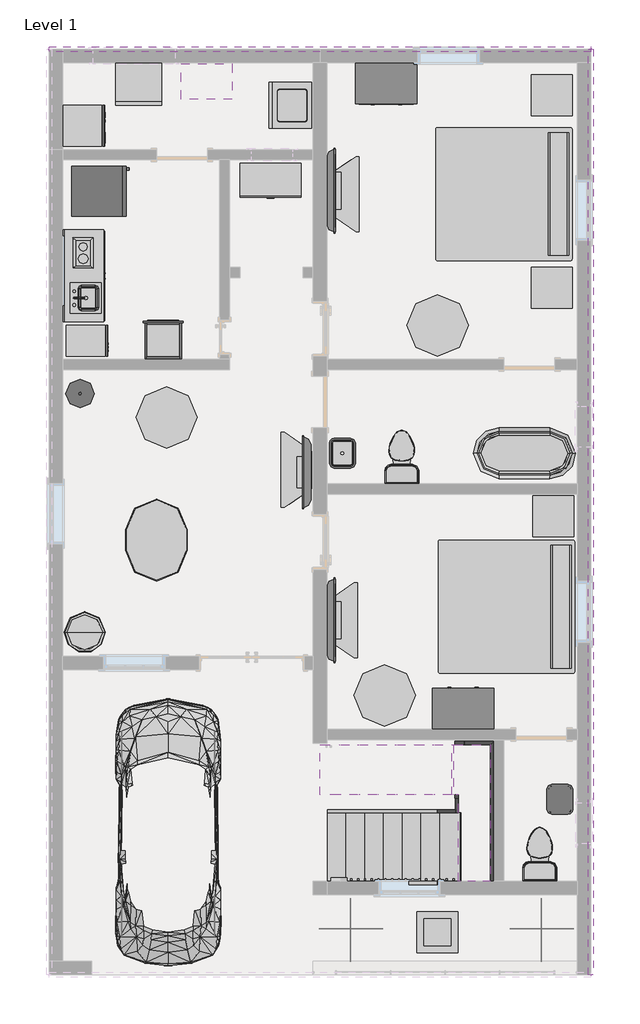
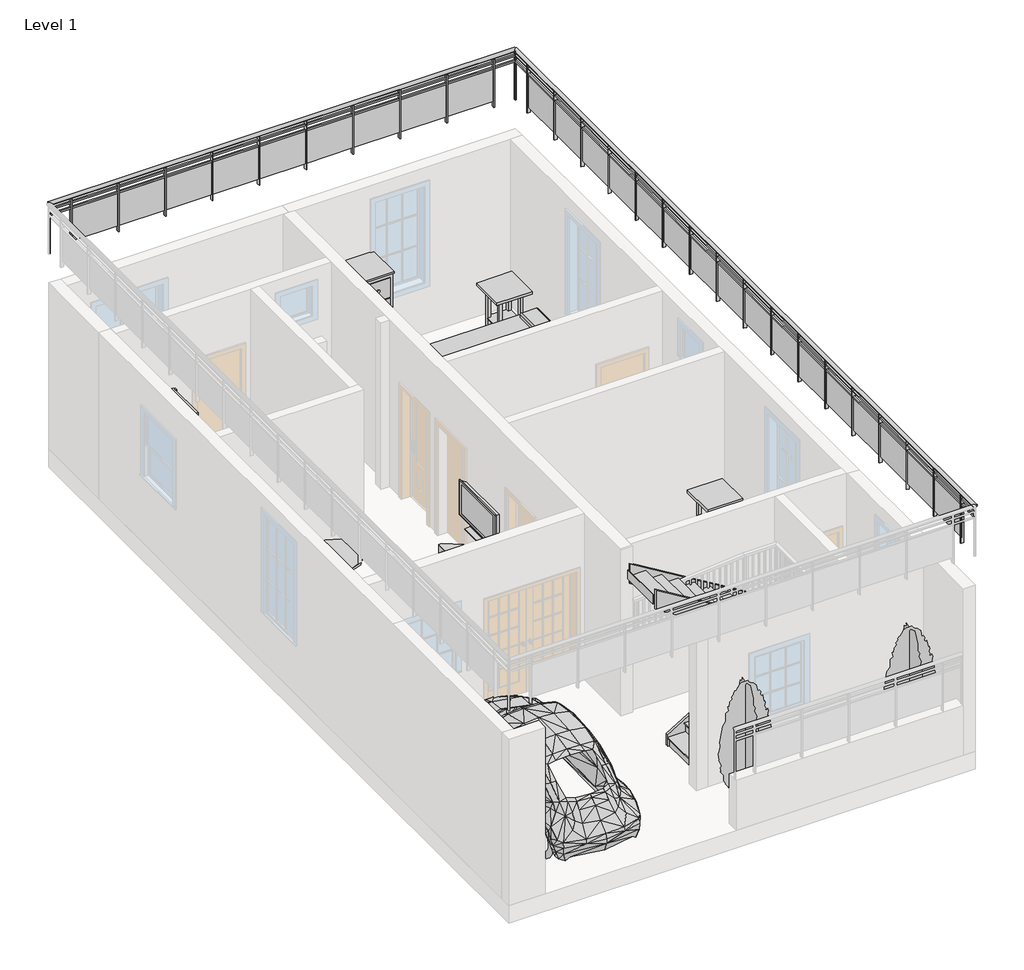
# One storey, part 3 of 3: 21 furniture elements, 9 proxies, 8 flow terminals, 8 members, 2 geographic elements, 2 railings, 2 stair flights, 1 slab.
"""IFC4 building model written with IfcOpenShell, lengths in millimetres."""

from ifc_helpers import new_model, si_unit, point, frame, origin, place, context, project, spatial, polyline, ellipse_curve, trimmed, outline, extrude, faceted_brep, transform, mapped, element, save
from ifc_brep_helpers import plane_surface, extruded_surface, advanced_brep
from components import proxy_7e1014cc, proxy_fe84b772, proxy_45b28599, proxy_b4d0e45e, proxy_844211aa, proxy_8b8c2dc4, rpc_beetle_rpc_beetle_3ce7ba48, proxy_a13a33b2, proxy_718fa39f, flow_terminal_871c2e40, flow_terminal_38af2918, flow_terminal_d49f872f, flow_terminal_62a433f7, toilet_domestic_3d_toilet_domestic_3d_f7549cf7, toilet_domestic_3d_toilet_domestic_3d_183bbd19, flow_terminal_b374fae2, furniture_1fc5af50, furniture_95afb093, furniture_33655958, furniture_e1dba61b, furniture_7a3aaa4f, furniture_fdf74506, tv_stand_tv_stand_6ce107e5, furniture_b5c51a22, furniture_be1c6672, furniture_905aceb5, furniture_4bee3317, furniture_5bc9ed15, furniture_a0cc3393, rpc_tree_conifer_chinese_juniper_7_1b9786cd, non_monolithic_landing_8c39f4e9, stair_flight_9de2ea67, stair_flight_c1e9d316

model = new_model("IFC4")

# Units and contexts
model_context = context("Model", 3, world=origin())
ifc_project = project(units=[si_unit("LENGTHUNIT", "METRE", prefix="MILLI")], contexts=[model_context])

# Site, building, storey
site = spatial("IfcSite", under=ifc_project)
building = spatial("IfcBuilding", under=site)
storey = spatial("IfcBuildingStorey", under=building, Name="Level 1", Elevation=0.0)

# Proxies
placement = place(None, origin())
proxy_shape = proxy_7e1014cc(model_context)
element("IfcBuildingElementProxy", 1, Name="18\" x 24\" x 34 1/2\"", ObjectType="18\" x 24\" x 34 1/2\"", at=placement, inside=storey, context=model_context, shape_type="MappedRepresentation", body=[
    mapped(proxy_shape, transform((-11751.937775, 7062.985832, 0.0), x_axis=(0.0, 1.0000000000000002, 0.0), y_axis=(-1.0000000000000002, 0.0, 0.0), z_axis=(0.0, 0.0, 1.0))),
])
proxy_2_shape = proxy_fe84b772(model_context)
element("IfcBuildingElementProxy", 2, Name="Cook Top-2 Unit : 12\" x 18\"", ObjectType="Cook Top-2 Unit : 12\" x 18\"", at=placement, inside=storey, context=model_context, shape_type="MappedRepresentation", body=[
    mapped(proxy_2_shape, transform((-11992.9873398, 8707.4280961, 0.0), x_axis=(-1.0, 0.0, 0.0), y_axis=(0.0, -1.0, 0.0), z_axis=(0.0, 0.0, 1.0))),
])
proxy_3_shape = proxy_45b28599(model_context)
element("IfcBuildingElementProxy", 3, Name="Dishwasher : 24\" x 24\" x 34\"", ObjectType="Dishwasher : 24\" x 24\" x 34\"", at=placement, inside=storey, context=model_context, shape_type="MappedRepresentation", body=[
    mapped(proxy_3_shape, transform((-11802.737775, 10187.185832, 0.0), x_axis=(0.0, 1.0000000000000002, 0.0), y_axis=(-1.0000000000000002, 0.0, 0.0), z_axis=(0.0, 0.0, 1.0))),
])
proxy_4_shape = proxy_b4d0e45e(model_context)
element("IfcBuildingElementProxy", 4, Name="Dryer : 27\" x 25\" x 35\"", ObjectType="Dryer : 27\" x 25\" x 35\"", at=placement, inside=storey, context=model_context, shape_type="MappedRepresentation", body=[
    mapped(proxy_4_shape, transform((-10864.6998835, 11506.4643043, 0.0), x_axis=(-1.0000000000000002, 0.0, 0.0), y_axis=(0.0, -1.0000000000000002, 0.0), z_axis=(0.0, 0.0, 1.0))),
])
proxy_5_shape = proxy_844211aa(model_context)
element("IfcBuildingElementProxy", 5, Name="Kitchenette - Small : 54\"", ObjectType="Kitchenette - Small : 54\"", at=placement, inside=storey, context=model_context, shape_type="MappedRepresentation", body=[
    mapped(proxy_5_shape, transform((-12373.9873398, 8315.5655956, 0.0), x_axis=(0.0, 1.0, 0.0), y_axis=(-1.0, 0.0, 0.0), z_axis=(0.0, 0.0, 1.0))),
])
proxy_6_shape = proxy_8b8c2dc4(model_context)
element("IfcBuildingElementProxy", 6, Name="Oven Double-Built-in : 21 1/2\" x 39 1/4\" x 21\"", ObjectType="Oven Double-Built-in : 21 1/2\" x 39 1/4\" x 21\"", at=placement, inside=storey, context=model_context, shape_type="MappedRepresentation", body=[
    mapped(proxy_6_shape, transform((-10910.5622671, 7510.1691595, 0.0), x_axis=(-1.0000000000000004, 0.0, 0.0), y_axis=(0.0, -1.0000000000000004, 0.0), z_axis=(0.0, 0.0, 1.0))),
])
rpc_beetle_rpc_beetle_shape = rpc_beetle_rpc_beetle_3ce7ba48(model_context)
element("IfcBuildingElementProxy", 7, Name="RPC Beetle : RPC Beetle", ObjectType="RPC Beetle : RPC Beetle", at=placement, inside=storey, context=model_context, shape_type="MappedRepresentation", body=[
    mapped(rpc_beetle_rpc_beetle_shape, transform((-10799.1873398, -1190.6966995, 0.0), x_axis=(1.0, 0.0, 0.0), y_axis=(0.0, 1.0, 0.0), z_axis=(0.0, 0.0, 1.0))),
])
proxy_7_shape = proxy_a13a33b2(model_context)
element("IfcBuildingElementProxy", 8, Name="Refrigerator : 30\" x 32\" RH", ObjectType="Refrigerator : 30\" x 32\" RH", at=placement, inside=storey, context=model_context, shape_type="MappedRepresentation", body=[
    mapped(proxy_7_shape, transform((-11848.5248398, 9596.754329, 0.0), x_axis=(0.0, 1.000000000000001, 0.0), y_axis=(-1.000000000000001, 0.0, 0.0), z_axis=(0.0, 0.0, 1.0))),
])
proxy_8_shape = proxy_718fa39f(model_context)
element("IfcBuildingElementProxy", 9, Name="Washer : 27\" x 25\" x 35\"", ObjectType="Washer : 27\" x 25\" x 35\"", at=placement, inside=storey, context=model_context, shape_type="MappedRepresentation", body=[
    mapped(proxy_8_shape, transform((-8703.937775, 10453.885832, 0.0), x_axis=(0.0, 1.000000000000002, 0.0), y_axis=(-1.000000000000002, 0.0, 0.0), z_axis=(0.0, 0.0, 1.0))),
])

# Flow terminals
flow_terminal_shape = flow_terminal_871c2e40(model_context)
element("IfcFlowTerminal", 10, ObjectType="Sink Kitchen-Island : 18\" x 18\"", at=placement, inside=storey, context=model_context, shape_type="MappedRepresentation", body=[
    mapped(flow_terminal_shape, transform((-12028.7419387, 7988.41406, 0.0), x_axis=(0.0, 1.0, 0.0), y_axis=(-1.0, 0.0, 0.0), z_axis=(0.0, 0.0, 1.0))),
])
flow_terminal_2_shape = flow_terminal_38af2918(model_context)
element("IfcFlowTerminal", 11, ObjectType="Sink Kitchen-Single : 30\" x 21\"", at=placement, inside=storey, context=model_context, shape_type="MappedRepresentation", body=[
    mapped(flow_terminal_2_shape, transform((-10243.3765804, 11227.5578994, 609.6), x_axis=(1.0, 0.0, 0.0), y_axis=(0.0, 1.0, 0.0), z_axis=(0.0, 0.0, 1.0))),
])
flow_terminal_3_shape = flow_terminal_d49f872f(model_context)
element("IfcFlowTerminal", 12, ObjectType="Sink Vanity-Round : 19\" x 19\"", at=placement, inside=storey, context=model_context, shape_type="MappedRepresentation", body=[
    mapped(flow_terminal_3_shape, transform((-12029.94095, 6485.05156, 609.6), x_axis=(0.0, 1.0000000000000002, 0.0), y_axis=(-1.0000000000000002, 0.0, 0.0), z_axis=(0.0, 0.0, 1.0))),
])
flow_terminal_4_shape = flow_terminal_62a433f7(model_context)
element("IfcFlowTerminal", 13, ObjectType="Sink Vanity-Square : 20\" x 18\"", at=placement, inside=storey, context=model_context, shape_type="MappedRepresentation", body=[
    mapped(flow_terminal_4_shape, transform((-8256.8419387, 5677.01406, 609.6), x_axis=(0.0, 1.0, 0.0), y_axis=(-1.0, 0.0, 0.0), z_axis=(0.0, 0.0, 1.0))),
])
element("IfcFlowTerminal", 14, ObjectType="Sink Vanity-Square : 20\" x 18\"", at=placement, inside=storey, context=model_context, shape_type="MappedRepresentation", body=[
    mapped(flow_terminal_4_shape, transform((-4908.7327409, 552.1925411, 609.6), x_axis=(0.0, -1.0000000000000004, 0.0), y_axis=(1.0000000000000004, 0.0, 0.0), z_axis=(0.0, 0.0, 1.0))),
])
toilet_domestic_3d_toilet_domestic_3d_shape = toilet_domestic_3d_toilet_domestic_3d_f7549cf7(model_context)
toilet_domestic_3d_toilet_domestic_3d_2_shape = toilet_domestic_3d_toilet_domestic_3d_183bbd19(model_context)
element("IfcFlowTerminal", 15, ObjectType="Toilet-Domestic-3D : Toilet-Domestic-3D", at=placement, inside=storey, context=model_context, shape_type="MappedRepresentation", body=[
    mapped(toilet_domestic_3d_toilet_domestic_3d_shape, transform((-5261.9873398, -188.0006721, 0.0), x_axis=(-0.9999999999999998, 0.0, 0.0), y_axis=(0.0, -0.9999999999999998, 0.0), z_axis=(0.0, 0.0, 1.0))),
    mapped(toilet_domestic_3d_toilet_domestic_3d_2_shape, transform((-5261.9873398, -188.0006721, 0.0), x_axis=(-0.9999999999999998, 0.0, 0.0), y_axis=(0.0, -0.9999999999999998, 0.0), z_axis=(0.0, 0.0, 1.0))),
])
element("IfcFlowTerminal", 16, ObjectType="Toilet-Domestic-3D : Toilet-Domestic-3D", at=placement, inside=storey, context=model_context, shape_type="MappedRepresentation", body=[
    mapped(toilet_domestic_3d_toilet_domestic_3d_shape, transform((-7319.3873398, 5730.1993279, 0.0), x_axis=(-1.0000000000000004, 0.0, 0.0), y_axis=(0.0, -1.0000000000000004, 0.0), z_axis=(0.0, 0.0, 1.0))),
    mapped(toilet_domestic_3d_toilet_domestic_3d_2_shape, transform((-7319.3873398, 5730.1993279, 0.0), x_axis=(-1.0000000000000004, 0.0, 0.0), y_axis=(0.0, -1.0000000000000004, 0.0), z_axis=(0.0, 0.0, 1.0))),
])
flow_terminal_5_shape = flow_terminal_b374fae2(model_context)
element("IfcFlowTerminal", 17, ObjectType="Tub-Free Standing-3D : 30\" x 60\"", at=placement, inside=storey, context=model_context, shape_type="MappedRepresentation", body=[
    mapped(flow_terminal_5_shape, transform((-5490.5873398, 5692.7033005, 0.0), x_axis=(0.0, -1.0, 0.0), y_axis=(1.0, 0.0, 0.0), z_axis=(0.0, 0.0, 1.0))),
])

# Furniture
furniture_shape = furniture_1fc5af50(model_context)
element("IfcFurniture", 18, ObjectType="Bed-Standard.0001 : King 78\" x 80\"", at=placement, inside=storey, context=model_context, shape_type="MappedRepresentation", body=[
    mapped(furniture_shape, transform((-5711.6922578, 3678.1918251, 0.0), x_axis=(0.0, -1.0, 0.0), y_axis=(1.0, 0.0, 0.0), z_axis=(0.0, 0.0, 1.0))),
])
element("IfcFurniture", 19, ObjectType="Bed-Standard.0001 : King 78\" x 80\"", at=placement, inside=storey, context=model_context, shape_type="MappedRepresentation", body=[
    mapped(furniture_shape, transform((-5749.7922578, 9824.9918251, 0.0), x_axis=(0.0, -1.0, 0.0), y_axis=(1.0, 0.0, 0.0), z_axis=(0.0, 0.0, 1.0))),
])
furniture_2_shape = furniture_95afb093(model_context)
element("IfcFurniture", 20, ObjectType="Counter Top w Sink Hole : 24\" Depth", at=placement, inside=storey, context=model_context, shape_type="MappedRepresentation", body=[
    mapped(furniture_2_shape, transform((-12373.9873398, 8848.9655956, 0.0), x_axis=(0.0, 1.0, 0.0), y_axis=(-1.0, 0.0, 0.0), z_axis=(0.0, 0.0, 1.0))),
])
furniture_3_shape = furniture_33655958(model_context)
element("IfcFurniture", 21, ObjectType="Dresser : 48\" x 72\" x 24\"", at=placement, inside=storey, context=model_context, shape_type="MappedRepresentation", body=[
    mapped(furniture_3_shape, transform((-6674.1805996, 1519.5403464, 0.0), x_axis=(-1.0000000000000004, 0.0, 0.0), y_axis=(0.0, -1.0000000000000004, 0.0), z_axis=(0.0, 0.0, 1.0))),
])
element("IfcFurniture", 22, ObjectType="Dresser : 48\" x 72\" x 24\"", at=placement, inside=storey, context=model_context, shape_type="MappedRepresentation", body=[
    mapped(furniture_3_shape, transform((-7278.79408, 11567.6662546, 0.0), x_axis=(1.0, 0.0, 0.0), y_axis=(0.0, 1.0, 0.0), z_axis=(0.0, 0.0, 1.0))),
])
furniture_4_shape = furniture_e1dba61b(model_context)
element("IfcFurniture", 23, ObjectType="Storage Pedestal : 20\" x 36\" x 36\"", at=placement, inside=storey, context=model_context, shape_type="MappedRepresentation", body=[
    mapped(furniture_4_shape, transform((-9095.1648259, 10691.0216766, 0.0), x_axis=(1.0, 0.0, 0.0), y_axis=(0.0, 1.0, 0.0), z_axis=(0.0, 0.0, 1.0))),
])
furniture_5_shape = furniture_7a3aaa4f(model_context)
element("IfcFurniture", 24, ObjectType="TV - Flat Screen : 42\"", at=placement, inside=storey, context=model_context, shape_type="MappedRepresentation", body=[
    mapped(furniture_5_shape, transform((-8732.4823155, 5404.2032892, 914.4), x_axis=(0.0, -1.0000000000000007, 0.0), y_axis=(1.0000000000000007, 0.0, 0.0), z_axis=(0.0, 0.0, 1.0))),
])
furniture_6_shape = furniture_fdf74506(model_context)
element("IfcFurniture", 25, ObjectType="TV - Flat Screen : 50\"", at=placement, inside=storey, context=model_context, shape_type="MappedRepresentation", body=[
    mapped(furniture_6_shape, transform((-8378.4487161, 3207.4478147, 914.4), x_axis=(0.0, 1.0000000000000002, 0.0), y_axis=(-1.0000000000000002, 0.0, 0.0), z_axis=(0.0, 0.0, 1.0))),
])
element("IfcFurniture", 26, ObjectType="TV - Flat Screen : 50\"", at=placement, inside=storey, context=model_context, shape_type="MappedRepresentation", body=[
    mapped(furniture_6_shape, transform((-8378.4487161, 9608.2478147, 914.4), x_axis=(0.0, 1.0000000000000002, 0.0), y_axis=(-1.0000000000000002, 0.0, 0.0), z_axis=(0.0, 0.0, 1.0))),
])
tv_stand_tv_stand_shape = tv_stand_tv_stand_6ce107e5(model_context)
element("IfcFurniture", 27, ObjectType="TV Stand : TV Stand", at=placement, inside=storey, context=model_context, shape_type="MappedRepresentation", body=[
    mapped(tv_stand_tv_stand_shape, transform((-8436.9873398, 3078.3152985, 0.0), x_axis=(0.0, 1.0000000000000002, 0.0), y_axis=(-1.0000000000000002, 0.0, 0.0), z_axis=(0.0, 0.0, 1.0))),
])
element("IfcFurniture", 28, ObjectType="TV Stand : TV Stand", at=placement, inside=storey, context=model_context, shape_type="MappedRepresentation", body=[
    mapped(tv_stand_tv_stand_shape, transform((-8411.5873398, 9428.3152985, 0.0), x_axis=(0.0, 1.0000000000000002, 0.0), y_axis=(-1.0000000000000002, 0.0, 0.0), z_axis=(0.0, 0.0, 1.0))),
])
element("IfcFurniture", 29, ObjectType="TV Stand : TV Stand", at=placement, inside=storey, context=model_context, shape_type="MappedRepresentation", body=[
    mapped(tv_stand_tv_stand_shape, transform((-8661.3692573, 5569.2377891, 0.0), x_axis=(0.0, -1.0000000000000007, 0.0), y_axis=(1.0000000000000007, 0.0, 0.0), z_axis=(0.0, 0.0, 1.0))),
])
furniture_7_shape = furniture_b5c51a22(model_context)
element("IfcFurniture", 30, ObjectType="Table-Coffee : 24\" x 24\" x 24\"", at=placement, inside=storey, context=model_context, shape_type="MappedRepresentation", body=[
    mapped(furniture_7_shape, transform((-6804.2531065, -1539.9077773, 0.0), x_axis=(1.0, 0.0, 0.0), y_axis=(0.0, 1.0, 0.0), z_axis=(0.0, 0.0, 1.0))),
])
furniture_8_shape = furniture_be1c6672(model_context)
element("IfcFurniture", 31, ObjectType="Table-Dining Oval : 36\" x 72\"", at=placement, inside=storey, context=model_context, shape_type="MappedRepresentation", body=[
    mapped(furniture_8_shape, transform((-11335.0857004, 4799.1229727, 0.0), x_axis=(0.0, 1.0000000000000002, 0.0), y_axis=(-1.0000000000000002, 0.0, 0.0), z_axis=(0.0, 0.0, 1.0))),
])
furniture_9_shape = furniture_905aceb5(model_context)
element("IfcFurniture", 32, ObjectType="Table-Dining Round w Chairs : 36\" Diameter", at=placement, inside=storey, context=model_context, shape_type="MappedRepresentation", body=[
    mapped(furniture_9_shape, transform((-10928.269307, 6410.9819891, 0.0), x_axis=(1.0, 0.0, 0.0), y_axis=(0.0, 1.0, 0.0), z_axis=(0.0, 0.0, 1.0))),
])
furniture_10_shape = furniture_4bee3317(model_context)
element("IfcFurniture", 33, ObjectType="Table-Ellipse : 72\" x 36\"", at=placement, inside=storey, context=model_context, shape_type="MappedRepresentation", body=[
    mapped(furniture_10_shape, transform((-6785.9873398, 7597.7033005, 0.0), x_axis=(1.0, 0.0, 0.0), y_axis=(0.0, 1.0, 0.0), z_axis=(0.0, 0.0, 1.0))),
])
element("IfcFurniture", 34, ObjectType="Table-Ellipse : 72\" x 36\"", at=placement, inside=storey, context=model_context, shape_type="MappedRepresentation", body=[
    mapped(furniture_10_shape, transform((-7573.3873398, 2085.9033005, 0.0), x_axis=(1.0, 0.0, 0.0), y_axis=(0.0, 1.0, 0.0), z_axis=(0.0, 0.0, 1.0))),
])
furniture_11_shape = furniture_5bc9ed15(model_context)
element("IfcFurniture", 35, ObjectType="Table-Night Stand : 24\" x 24\" x 30\"", at=placement, inside=storey, context=model_context, shape_type="MappedRepresentation", body=[
    mapped(furniture_11_shape, transform((-5367.3209701, 4448.1033005, 0.0), x_axis=(1.0, 0.0, 0.0), y_axis=(0.0, 1.0, 0.0), z_axis=(0.0, 0.0, 1.0))),
])
element("IfcFurniture", 36, ObjectType="Table-Night Stand : 24\" x 24\" x 30\"", at=placement, inside=storey, context=model_context, shape_type="MappedRepresentation", body=[
    mapped(furniture_11_shape, transform((-5392.7209701, 10721.9033005, 0.0), x_axis=(1.0, 0.0, 0.0), y_axis=(0.0, 1.0, 0.0), z_axis=(0.0, 0.0, 1.0))),
])
element("IfcFurniture", 37, ObjectType="Table-Night Stand : 24\" x 24\" x 30\"", at=placement, inside=storey, context=model_context, shape_type="MappedRepresentation", body=[
    mapped(furniture_11_shape, transform((-5392.7209701, 7851.7033005, 0.0), x_axis=(1.0, 0.0, 0.0), y_axis=(0.0, 1.0, 0.0), z_axis=(0.0, 0.0, 1.0))),
])
furniture_12_shape = furniture_a0cc3393(model_context)
element("IfcFurniture", 38, ObjectType="Table-Round : 36\" Diameter", at=placement, inside=storey, context=model_context, shape_type="MappedRepresentation", body=[
    mapped(furniture_12_shape, transform((-12043.7873398, 3025.7033005, 0.0), x_axis=(1.0, 0.0, 0.0), y_axis=(0.0, 1.0, 0.0), z_axis=(0.0, 0.0, 1.0))),
])

# Geographic elements
rpc_tree_conifer_chinese_juniper_7_shape = rpc_tree_conifer_chinese_juniper_7_1b9786cd(model_context)
element("IfcGeographicElement", 39, ObjectType="RPC Tree - Conifer : Chinese Juniper - 7'", at=placement, inside=storey, context=model_context, shape_type="MappedRepresentation", body=[
    mapped(rpc_tree_conifer_chinese_juniper_7_shape, transform((-5236.7840109, -1393.8966995, 0.0), x_axis=(1.0, 0.0, 0.0), y_axis=(0.0, 1.0, 0.0), z_axis=(0.0, 0.0, 1.0))),
])
element("IfcGeographicElement", 40, ObjectType="RPC Tree - Conifer : Chinese Juniper - 7'", at=placement, inside=storey, context=model_context, shape_type="MappedRepresentation", body=[
    mapped(rpc_tree_conifer_chinese_juniper_7_shape, transform((-8081.5840109, -1393.8966995, 0.0), x_axis=(1.0, 0.0, 0.0), y_axis=(0.0, 1.0, 0.0), z_axis=(0.0, 0.0, 1.0))),
])

# Members
element("IfcMember", 41, ObjectType="Stringer - 2\" Width", at=placement, inside=storey, context=model_context, shape_type="SweptSolid", body=[
    extrude(outline(polyline([(1164.1905989, -6470.7655018), (1520.5993604, -6470.7655018), (2752.114512, -8502.7655018), (2395.7057504, -8502.7655018), (1164.1905989, -6470.7655018)])), frame((0.0, 551.195692, 0.0), z_axis=(0.0, 1.0, 0.0), x_axis=(0.0, 0.0, 1.0)), (0.0, 0.0, 1.0), 50.8),
])
element("IfcMember", 42, ObjectType="Stringer - 2\" Width", at=placement, inside=storey, context=model_context, shape_type="SweptSolid", body=[
    extrude(outline(polyline([(1126.0666667, -6407.8610136), (1430.8666667, -6322.7065571), (2752.114512, -8502.7655018), (2395.7057504, -8502.7655018), (1126.0666667, -6407.8610136)])), frame((0.0, 1348.8576368, 0.0), z_axis=(0.0, 1.0, 0.0), x_axis=(0.0, 0.0, 1.0)), (0.0, 0.0, 1.0), 50.8),
])
element("IfcMember", 43, ObjectType="Stringer - 2\" Width", at=placement, inside=storey, context=model_context, shape_type="SweptSolid", body=[
    extrude(outline(polyline([(212.114512, -8426.5655018), (0.0, -8426.5655018), (0.0, -8188.47999), (1010.251205, -6521.5655018), (1366.6599665, -6521.5655018), (212.114512, -8426.5655018)])), frame((0.0, 332.8576368, 0.0), z_axis=(0.0, 1.0, 0.0), x_axis=(0.0, 0.0, 1.0)), (0.0, 0.0, 1.0), 50.8),
])
element("IfcMember", 44, ObjectType="Stringer - 2\" Width", at=placement, inside=storey, context=model_context, shape_type="SweptSolid", body=[
    extrude(outline(polyline([(212.114512, -8426.5655018), (0.0, -8426.5655018), (0.0, -8188.47999), (1126.0666667, -6330.46999), (1430.8666667, -6415.6244466), (212.114512, -8426.5655018)])), frame((0.0, -733.4966995, 0.0), z_axis=(0.0, 1.0, 0.0), x_axis=(0.0, 0.0, 1.0)), (0.0, 0.0, 1.0), 50.8),
])
element("IfcMember", 45, ObjectType="Stringer - 2\" Width", at=placement, inside=storey, context=model_context, shape_type="SweptSolid", body=[
    extrude(outline(polyline([(-6521.5655018, 551.195692), (-6470.7655018, 551.195692), (-6470.7655018, 332.8576368), (-6521.5655018, 332.8576368), (-6521.5655018, 551.195692)])), frame((0.0, 0.0, 1126.0666667), z_axis=(0.0, 0.0, 1.0), x_axis=(1.0, 0.0, 0.0)), (0.0, 0.0, 1.0), 304.8),
])
element("IfcMember", 46, ObjectType="Stringer - 2\" Width", at=placement, inside=storey, context=model_context, shape_type="Brep", body=[
    faceted_brep([(-6415.6244466, -682.6966995, 1430.8666667), (-6415.6244466, -733.4966995, 1430.8666667), (-5948.7047162, -733.4966995, 1430.8666667), (-5999.5047162, -682.6966995, 1430.8666667), (-6330.46999, -682.6966995, 1126.0666667), (-5999.5047162, -682.6966995, 1126.0666667), (-6330.46999, -733.4966995, 1126.0666667), (-5948.7047162, -733.4966995, 1126.0666667)], [[[0, 1, 2, 3]], [[4, 0, 3, 5]], [[6, 4, 5, 7]], [[1, 6, 7, 2]], [[1, 0, 4, 6]], [[2, 7, 5, 3]]]),
])
element("IfcMember", 47, ObjectType="Stringer - 2\" Width", at=placement, inside=storey, context=model_context, shape_type="SweptSolid", body=[
    extrude(outline(polyline([(-5948.7047162, -733.4966995), (-5999.5047162, -682.6966995), (-5999.5047162, 1348.8576368), (-5948.7047162, 1399.6576368), (-5948.7047162, -733.4966995)])), frame((0.0, 0.0, 1126.0666667), z_axis=(0.0, 0.0, 1.0), x_axis=(1.0, 0.0, 0.0)), (0.0, 0.0, 1.0), 304.8),
])
element("IfcMember", 48, ObjectType="Stringer - 2\" Width", at=placement, inside=storey, context=model_context, shape_type="Brep", body=[
    faceted_brep([(-5999.5047162, 1348.8576368, 1430.8666667), (-5948.7047162, 1399.6576368, 1430.8666667), (-6322.7065571, 1399.6576368, 1430.8666667), (-6322.7065571, 1348.8576368, 1430.8666667), (-5999.5047162, 1348.8576368, 1126.0666667), (-6407.8610136, 1348.8576368, 1126.0666667), (-5948.7047162, 1399.6576368, 1126.0666667), (-6407.8610136, 1399.6576368, 1126.0666667)], [[[0, 1, 2, 3]], [[4, 0, 3, 5]], [[6, 4, 5, 7]], [[1, 6, 7, 2]], [[1, 0, 4, 6]], [[2, 7, 5, 3]]]),
])

# Railings
element("IfcRailing", 49, ObjectType="Glass Panel - Bottom Fill", at=placement, inside=storey, context=model_context, shape_type="SolidModel", body=[
    advanced_brep(
    [(-4499.9873398, 11674.4033005, 4495.8), (-4499.9873398, 11750.6033005, 4495.8), (-12577.1873398, 11674.4033005, 4495.8), (-12577.1873398, 11750.6033005, 4495.8)],
    [
        (0, 1, ellipse_curve(frame((-4499.9873398, 11712.5033005, 4495.8), z_axis=(1.0, 0.0, 0.0), x_axis=(0.0, 1.0, 0.0)), 38.1, 28.575)),
        (1, 0, ellipse_curve(frame((-4499.9873398, 11712.5033005, 4495.8), z_axis=(1.0, 0.0, 0.0), x_axis=(0.0, 1.0, 0.0)), 38.1, 28.575)),
        (2, 3, ellipse_curve(frame((-12577.1873398, 11712.5033005, 4495.8), z_axis=(-1.0, 0.0, 0.0), x_axis=(0.0, 1.0, 0.0)), 38.1, 28.575)),
        (3, 2, ellipse_curve(frame((-12577.1873398, 11712.5033005, 4495.8), z_axis=(-1.0, 0.0, 0.0), x_axis=(0.0, 1.0, 0.0)), 38.1, 28.575)),
        (0, 2),
        (3, 1),
    ],
    [
        plane_surface(frame((-4499.9873398, 11712.5033005, 4495.8), z_axis=(1.0, 0.0, 0.0), x_axis=(0.0, -1.0, 0.0))),
        plane_surface(frame((-12577.1873398, 11712.5033005, 4495.8), z_axis=(-1.0, 0.0, 0.0), x_axis=(0.0, -1.0, 0.0))),
        extruded_surface(trimmed(ellipse_curve(frame((-12577.1873398, 11712.5033005, 4495.8), z_axis=(1.0, 0.0, 0.0), x_axis=(0.0, 1.0, 0.0)), 38.1, 28.575), [point((-12577.1873398, 11674.4033005, 4495.8))], [point((-12577.1873398, 11750.6033005, 4495.8))], True, "CARTESIAN"), (8077.200000000001, 0.0, 0.0), 8077.200000000001),
        extruded_surface(trimmed(ellipse_curve(frame((-12577.1873398, 11712.5033005, 4495.8), z_axis=(1.0, 0.0, 0.0), x_axis=(0.0, 1.0, 0.0)), 38.1, 28.575), [point((-12577.1873398, 11750.6033005, 4495.8))], [point((-12577.1873398, 11674.4033005, 4495.8))], True, "CARTESIAN"), (8077.200000000001, 0.0, 0.0), 8077.200000000001),
    ],
    [
        (0, [[1, 2]]),
        (1, [[3, 4]]),
        (2, [[-1, 5, -4, 6]]),
        (3, [[-2, -6, -3, -5]]),
    ],
),
    extrude(outline(polyline([(-4499.9873398, 11725.2033005), (-4499.9873398, 11699.8033005), (-12577.1873398, 11699.8033005), (-12577.1873398, 11725.2033005), (-4499.9873398, 11725.2033005)])), frame((0.0, 0.0, 4381.5), z_axis=(0.0, 0.0, 1.0), x_axis=(1.0, 0.0, 0.0)), (0.0, 0.0, 1.0), 25.4),
    extrude(outline(polyline([(-4499.9873398, 11725.2033005), (-4499.9873398, 11699.8033005), (-12577.1873398, 11699.8033005), (-12577.1873398, 11725.2033005), (-4499.9873398, 11725.2033005)])), frame((0.0, 0.0, 4279.9), z_axis=(0.0, 0.0, 1.0), x_axis=(1.0, 0.0, 0.0)), (0.0, 0.0, 1.0), 25.4),
    extrude(outline(polyline([(-12189.8373398, 11737.9033005), (-12189.8373398, 11687.1033005), (-12202.5373398, 11687.1033005), (-12202.5373398, 11737.9033005), (-12189.8373398, 11737.9033005)])), frame((0.0, 0.0, 3581.4), z_axis=(0.0, 0.0, 1.0), x_axis=(1.0, 0.0, 0.0)), (0.0, 0.0, 1.0), 885.6788223),
    extrude(outline(polyline([(-11383.3873398, 11705.9681435), (-12196.1873398, 11705.9681435), (-12196.1873398, 11712.3181435), (-11383.3873398, 11712.3181435), (-11383.3873398, 11705.9681435)])), frame((0.0, 0.0, 3683.0), z_axis=(0.0, 0.0, 1.0), x_axis=(1.0, 0.0, 0.0)), (0.0, 0.0, 1.0), 596.9),
    extrude(outline(polyline([(-11377.0373398, 11737.9033005), (-11377.0373398, 11687.1033005), (-11389.7373398, 11687.1033005), (-11389.7373398, 11737.9033005), (-11377.0373398, 11737.9033005)])), frame((0.0, 0.0, 3581.4), z_axis=(0.0, 0.0, 1.0), x_axis=(1.0, 0.0, 0.0)), (0.0, 0.0, 1.0), 885.6788223),
    extrude(outline(polyline([(-10570.5873398, 11705.9681435), (-11383.3873398, 11705.9681435), (-11383.3873398, 11712.3181435), (-10570.5873398, 11712.3181435), (-10570.5873398, 11705.9681435)])), frame((0.0, 0.0, 3683.0), z_axis=(0.0, 0.0, 1.0), x_axis=(1.0, 0.0, 0.0)), (0.0, 0.0, 1.0), 596.9),
    extrude(outline(polyline([(-10564.2373398, 11737.9033005), (-10564.2373398, 11687.1033005), (-10576.9373398, 11687.1033005), (-10576.9373398, 11737.9033005), (-10564.2373398, 11737.9033005)])), frame((0.0, 0.0, 3581.4), z_axis=(0.0, 0.0, 1.0), x_axis=(1.0, 0.0, 0.0)), (0.0, 0.0, 1.0), 885.6788223),
    extrude(outline(polyline([(-9757.7873398, 11705.9681435), (-10570.5873398, 11705.9681435), (-10570.5873398, 11712.3181435), (-9757.7873398, 11712.3181435), (-9757.7873398, 11705.9681435)])), frame((0.0, 0.0, 3683.0), z_axis=(0.0, 0.0, 1.0), x_axis=(1.0, 0.0, 0.0)), (0.0, 0.0, 1.0), 596.9),
    extrude(outline(polyline([(-9751.4373398, 11737.9033005), (-9751.4373398, 11687.1033005), (-9764.1373398, 11687.1033005), (-9764.1373398, 11737.9033005), (-9751.4373398, 11737.9033005)])), frame((0.0, 0.0, 3581.4), z_axis=(0.0, 0.0, 1.0), x_axis=(1.0, 0.0, 0.0)), (0.0, 0.0, 1.0), 885.6788223),
    extrude(outline(polyline([(-8944.9873398, 11705.9681435), (-9757.7873398, 11705.9681435), (-9757.7873398, 11712.3181435), (-8944.9873398, 11712.3181435), (-8944.9873398, 11705.9681435)])), frame((0.0, 0.0, 3683.0), z_axis=(0.0, 0.0, 1.0), x_axis=(1.0, 0.0, 0.0)), (0.0, 0.0, 1.0), 596.9),
    extrude(outline(polyline([(-8938.6373398, 11737.9033005), (-8938.6373398, 11687.1033005), (-8951.3373398, 11687.1033005), (-8951.3373398, 11737.9033005), (-8938.6373398, 11737.9033005)])), frame((0.0, 0.0, 3581.4), z_axis=(0.0, 0.0, 1.0), x_axis=(1.0, 0.0, 0.0)), (0.0, 0.0, 1.0), 885.6788223),
    extrude(outline(polyline([(-8132.1873398, 11705.9681435), (-8944.9873398, 11705.9681435), (-8944.9873398, 11712.3181435), (-8132.1873398, 11712.3181435), (-8132.1873398, 11705.9681435)])), frame((0.0, 0.0, 3683.0), z_axis=(0.0, 0.0, 1.0), x_axis=(1.0, 0.0, 0.0)), (0.0, 0.0, 1.0), 596.9),
    extrude(outline(polyline([(-8125.8373398, 11737.9033005), (-8125.8373398, 11687.1033005), (-8138.5373398, 11687.1033005), (-8138.5373398, 11737.9033005), (-8125.8373398, 11737.9033005)])), frame((0.0, 0.0, 3581.4), z_axis=(0.0, 0.0, 1.0), x_axis=(1.0, 0.0, 0.0)), (0.0, 0.0, 1.0), 885.6788223),
    extrude(outline(polyline([(-7319.3873398, 11705.9681435), (-8132.1873398, 11705.9681435), (-8132.1873398, 11712.3181435), (-7319.3873398, 11712.3181435), (-7319.3873398, 11705.9681435)])), frame((0.0, 0.0, 3683.0), z_axis=(0.0, 0.0, 1.0), x_axis=(1.0, 0.0, 0.0)), (0.0, 0.0, 1.0), 596.9),
    extrude(outline(polyline([(-7313.0373398, 11737.9033005), (-7313.0373398, 11687.1033005), (-7325.7373398, 11687.1033005), (-7325.7373398, 11737.9033005), (-7313.0373398, 11737.9033005)])), frame((0.0, 0.0, 3581.4), z_axis=(0.0, 0.0, 1.0), x_axis=(1.0, 0.0, 0.0)), (0.0, 0.0, 1.0), 885.6788223),
    extrude(outline(polyline([(-6506.5873398, 11705.9681435), (-7319.3873398, 11705.9681435), (-7319.3873398, 11712.3181435), (-6506.5873398, 11712.3181435), (-6506.5873398, 11705.9681435)])), frame((0.0, 0.0, 3683.0), z_axis=(0.0, 0.0, 1.0), x_axis=(1.0, 0.0, 0.0)), (0.0, 0.0, 1.0), 596.9),
    extrude(outline(polyline([(-6500.2373398, 11737.9033005), (-6500.2373398, 11687.1033005), (-6512.9373398, 11687.1033005), (-6512.9373398, 11737.9033005), (-6500.2373398, 11737.9033005)])), frame((0.0, 0.0, 3581.4), z_axis=(0.0, 0.0, 1.0), x_axis=(1.0, 0.0, 0.0)), (0.0, 0.0, 1.0), 885.6788223),
    extrude(outline(polyline([(-5693.7873398, 11705.9681435), (-6506.5873398, 11705.9681435), (-6506.5873398, 11712.3181435), (-5693.7873398, 11712.3181435), (-5693.7873398, 11705.9681435)])), frame((0.0, 0.0, 3683.0), z_axis=(0.0, 0.0, 1.0), x_axis=(1.0, 0.0, 0.0)), (0.0, 0.0, 1.0), 596.9),
    extrude(outline(polyline([(-5687.4373398, 11737.9033005), (-5687.4373398, 11687.1033005), (-5700.1373398, 11687.1033005), (-5700.1373398, 11737.9033005), (-5687.4373398, 11737.9033005)])), frame((0.0, 0.0, 3581.4), z_axis=(0.0, 0.0, 1.0), x_axis=(1.0, 0.0, 0.0)), (0.0, 0.0, 1.0), 885.6788223),
    extrude(outline(polyline([(-4880.9873398, 11705.9681435), (-5693.7873398, 11705.9681435), (-5693.7873398, 11712.3181435), (-4880.9873398, 11712.3181435), (-4880.9873398, 11705.9681435)])), frame((0.0, 0.0, 3683.0), z_axis=(0.0, 0.0, 1.0), x_axis=(1.0, 0.0, 0.0)), (0.0, 0.0, 1.0), 596.9),
    extrude(outline(polyline([(-4874.6373398, 11737.9033005), (-4874.6373398, 11687.1033005), (-4887.3373398, 11687.1033005), (-4887.3373398, 11737.9033005), (-4874.6373398, 11737.9033005)])), frame((0.0, 0.0, 3581.4), z_axis=(0.0, 0.0, 1.0), x_axis=(1.0, 0.0, 0.0)), (0.0, 0.0, 1.0), 885.6788223),
    extrude(outline(polyline([(-12564.4873398, 11722.0283005), (-12564.4873398, 11702.9783005), (-12583.5373398, 11702.9783005), (-12583.5373398, 11722.0283005), (-12564.4873398, 11722.0283005)])), frame((0.0, 0.0, 3581.4), z_axis=(0.0, 0.0, 1.0), x_axis=(1.0, 0.0, 0.0)), (0.0, 0.0, 1.0), 885.6788223),
    extrude(outline(polyline([(-4493.6373398, 11722.0283005), (-4493.6373398, 11702.9783005), (-4512.6873398, 11702.9783005), (-4512.6873398, 11722.0283005), (-4493.6373398, 11722.0283005)])), frame((0.0, 0.0, 3581.4), z_axis=(0.0, 0.0, 1.0), x_axis=(1.0, 0.0, 0.0)), (0.0, 0.0, 1.0), 885.6788223),
])
element("IfcRailing", 50, ObjectType="Glass Panel - Bottom Fill", at=placement, inside=storey, context=model_context, shape_type="SolidModel", body=[
    advanced_brep(
    [(-4538.0873398, -2079.6966995, 4495.8), (-4461.8873398, -2079.6966995, 4495.8), (-4538.0873398, 11712.5033005, 4495.8), (-4461.8873398, 11712.5033005, 4495.8)],
    [
        (0, 1, ellipse_curve(frame((-4499.9873398, -2079.6966995, 4495.8), z_axis=(0.0, -1.0, 0.0), x_axis=(1.0, 0.0, 0.0)), 38.1, 28.575)),
        (1, 0, ellipse_curve(frame((-4499.9873398, -2079.6966995, 4495.8), z_axis=(0.0, -1.0, 0.0), x_axis=(1.0, 0.0, 0.0)), 38.1, 28.575)),
        (2, 3, ellipse_curve(frame((-4499.9873398, 11712.5033005, 4495.8), z_axis=(0.0, 1.0, 0.0), x_axis=(1.0, 0.0, 0.0)), 38.1, 28.575)),
        (3, 2, ellipse_curve(frame((-4499.9873398, 11712.5033005, 4495.8), z_axis=(0.0, 1.0, 0.0), x_axis=(1.0, 0.0, 0.0)), 38.1, 28.575)),
        (0, 2),
        (3, 1),
    ],
    [
        plane_surface(frame((-4499.9873398, -2079.6966995, 4495.8), z_axis=(0.0, -1.0, 0.0), x_axis=(0.0, 0.0, 1.0))),
        plane_surface(frame((-4499.9873398, 11712.5033005, 4495.8), z_axis=(0.0, 1.0, 0.0), x_axis=(0.0, 0.0, 1.0))),
        extruded_surface(trimmed(ellipse_curve(frame((-4499.9873398, 11712.5033005, 4495.8), z_axis=(0.0, -1.0, 0.0), x_axis=(1.0, 0.0, 0.0)), 38.1, 28.575), [point((-4538.0873398, 11712.5033005, 4495.8))], [point((-4461.8873398, 11712.5033005, 4495.8))], True, "CARTESIAN"), (0.0, -13792.2, 0.0), 13792.2),
        extruded_surface(trimmed(ellipse_curve(frame((-4499.9873398, 11712.5033005, 4495.8), z_axis=(0.0, -1.0, 0.0), x_axis=(1.0, 0.0, 0.0)), 38.1, 28.575), [point((-4461.8873398, 11712.5033005, 4495.8))], [point((-4538.0873398, 11712.5033005, 4495.8))], True, "CARTESIAN"), (0.0, -13792.2, 0.0), 13792.2),
    ],
    [
        (0, [[1, 2]]),
        (1, [[3, 4]]),
        (2, [[-1, 5, -4, 6]]),
        (3, [[-2, -6, -3, -5]]),
    ],
),
    extrude(outline(polyline([(-4487.2873398, -2079.6966995), (-4512.6873398, -2079.6966995), (-4512.6873398, 11712.5033005), (-4487.2873398, 11712.5033005), (-4487.2873398, -2079.6966995)])), frame((0.0, 0.0, 4381.5), z_axis=(0.0, 0.0, 1.0), x_axis=(1.0, 0.0, 0.0)), (0.0, 0.0, 1.0), 25.4),
    extrude(outline(polyline([(-4487.2873398, -2079.6966995), (-4512.6873398, -2079.6966995), (-4512.6873398, 11712.5033005), (-4487.2873398, 11712.5033005), (-4487.2873398, -2079.6966995)])), frame((0.0, 0.0, 4279.9), z_axis=(0.0, 0.0, 1.0), x_axis=(1.0, 0.0, 0.0)), (0.0, 0.0, 1.0), 25.4),
    extrude(outline(polyline([(-4474.5873398, 11312.4533005), (-4525.3873398, 11312.4533005), (-4525.3873398, 11325.1533005), (-4474.5873398, 11325.1533005), (-4474.5873398, 11312.4533005)])), frame((0.0, 0.0, 3581.4), z_axis=(0.0, 0.0, 1.0), x_axis=(1.0, 0.0, 0.0)), (0.0, 0.0, 1.0), 885.6788223),
    extrude(outline(polyline([(-4506.5224968, 10506.0033005), (-4506.5224968, 11318.8033005), (-4500.1724968, 11318.8033005), (-4500.1724968, 10506.0033005), (-4506.5224968, 10506.0033005)])), frame((0.0, 0.0, 3683.0), z_axis=(0.0, 0.0, 1.0), x_axis=(1.0, 0.0, 0.0)), (0.0, 0.0, 1.0), 596.9),
    extrude(outline(polyline([(-4474.5873398, 10499.6533005), (-4525.3873398, 10499.6533005), (-4525.3873398, 10512.3533005), (-4474.5873398, 10512.3533005), (-4474.5873398, 10499.6533005)])), frame((0.0, 0.0, 3581.4), z_axis=(0.0, 0.0, 1.0), x_axis=(1.0, 0.0, 0.0)), (0.0, 0.0, 1.0), 885.6788223),
    extrude(outline(polyline([(-4506.5224968, 9693.2033005), (-4506.5224968, 10506.0033005), (-4500.1724968, 10506.0033005), (-4500.1724968, 9693.2033005), (-4506.5224968, 9693.2033005)])), frame((0.0, 0.0, 3683.0), z_axis=(0.0, 0.0, 1.0), x_axis=(1.0, 0.0, 0.0)), (0.0, 0.0, 1.0), 596.9),
    extrude(outline(polyline([(-4474.5873398, 9686.8533005), (-4525.3873398, 9686.8533005), (-4525.3873398, 9699.5533005), (-4474.5873398, 9699.5533005), (-4474.5873398, 9686.8533005)])), frame((0.0, 0.0, 3581.4), z_axis=(0.0, 0.0, 1.0), x_axis=(1.0, 0.0, 0.0)), (0.0, 0.0, 1.0), 885.6788223),
    extrude(outline(polyline([(-4506.5224968, 8880.4033005), (-4506.5224968, 9693.2033005), (-4500.1724968, 9693.2033005), (-4500.1724968, 8880.4033005), (-4506.5224968, 8880.4033005)])), frame((0.0, 0.0, 3683.0), z_axis=(0.0, 0.0, 1.0), x_axis=(1.0, 0.0, 0.0)), (0.0, 0.0, 1.0), 596.9),
    extrude(outline(polyline([(-4474.5873398, 8874.0533005), (-4525.3873398, 8874.0533005), (-4525.3873398, 8886.7533005), (-4474.5873398, 8886.7533005), (-4474.5873398, 8874.0533005)])), frame((0.0, 0.0, 3581.4), z_axis=(0.0, 0.0, 1.0), x_axis=(1.0, 0.0, 0.0)), (0.0, 0.0, 1.0), 885.6788223),
    extrude(outline(polyline([(-4506.5224968, 8067.6033005), (-4506.5224968, 8880.4033005), (-4500.1724968, 8880.4033005), (-4500.1724968, 8067.6033005), (-4506.5224968, 8067.6033005)])), frame((0.0, 0.0, 3683.0), z_axis=(0.0, 0.0, 1.0), x_axis=(1.0, 0.0, 0.0)), (0.0, 0.0, 1.0), 596.9),
    extrude(outline(polyline([(-4474.5873398, 8061.2533005), (-4525.3873398, 8061.2533005), (-4525.3873398, 8073.9533005), (-4474.5873398, 8073.9533005), (-4474.5873398, 8061.2533005)])), frame((0.0, 0.0, 3581.4), z_axis=(0.0, 0.0, 1.0), x_axis=(1.0, 0.0, 0.0)), (0.0, 0.0, 1.0), 885.6788223),
    extrude(outline(polyline([(-4506.5224968, 7254.8033005), (-4506.5224968, 8067.6033005), (-4500.1724968, 8067.6033005), (-4500.1724968, 7254.8033005), (-4506.5224968, 7254.8033005)])), frame((0.0, 0.0, 3683.0), z_axis=(0.0, 0.0, 1.0), x_axis=(1.0, 0.0, 0.0)), (0.0, 0.0, 1.0), 596.9),
    extrude(outline(polyline([(-4474.5873398, 7248.4533005), (-4525.3873398, 7248.4533005), (-4525.3873398, 7261.1533005), (-4474.5873398, 7261.1533005), (-4474.5873398, 7248.4533005)])), frame((0.0, 0.0, 3581.4), z_axis=(0.0, 0.0, 1.0), x_axis=(1.0, 0.0, 0.0)), (0.0, 0.0, 1.0), 885.6788223),
    extrude(outline(polyline([(-4506.5224968, 6442.0033005), (-4506.5224968, 7254.8033005), (-4500.1724968, 7254.8033005), (-4500.1724968, 6442.0033005), (-4506.5224968, 6442.0033005)])), frame((0.0, 0.0, 3683.0), z_axis=(0.0, 0.0, 1.0), x_axis=(1.0, 0.0, 0.0)), (0.0, 0.0, 1.0), 596.9),
    extrude(outline(polyline([(-4474.5873398, 6435.6533005), (-4525.3873398, 6435.6533005), (-4525.3873398, 6448.3533005), (-4474.5873398, 6448.3533005), (-4474.5873398, 6435.6533005)])), frame((0.0, 0.0, 3581.4), z_axis=(0.0, 0.0, 1.0), x_axis=(1.0, 0.0, 0.0)), (0.0, 0.0, 1.0), 885.6788223),
    extrude(outline(polyline([(-4506.5224968, 5629.2033005), (-4506.5224968, 6442.0033005), (-4500.1724968, 6442.0033005), (-4500.1724968, 5629.2033005), (-4506.5224968, 5629.2033005)])), frame((0.0, 0.0, 3683.0), z_axis=(0.0, 0.0, 1.0), x_axis=(1.0, 0.0, 0.0)), (0.0, 0.0, 1.0), 596.9),
    extrude(outline(polyline([(-4474.5873398, 5622.8533005), (-4525.3873398, 5622.8533005), (-4525.3873398, 5635.5533005), (-4474.5873398, 5635.5533005), (-4474.5873398, 5622.8533005)])), frame((0.0, 0.0, 3581.4), z_axis=(0.0, 0.0, 1.0), x_axis=(1.0, 0.0, 0.0)), (0.0, 0.0, 1.0), 885.6788223),
    extrude(outline(polyline([(-4506.5224968, 4816.4033005), (-4506.5224968, 5629.2033005), (-4500.1724968, 5629.2033005), (-4500.1724968, 4816.4033005), (-4506.5224968, 4816.4033005)])), frame((0.0, 0.0, 3683.0), z_axis=(0.0, 0.0, 1.0), x_axis=(1.0, 0.0, 0.0)), (0.0, 0.0, 1.0), 596.9),
    extrude(outline(polyline([(-4474.5873398, 4810.0533005), (-4525.3873398, 4810.0533005), (-4525.3873398, 4822.7533005), (-4474.5873398, 4822.7533005), (-4474.5873398, 4810.0533005)])), frame((0.0, 0.0, 3581.4), z_axis=(0.0, 0.0, 1.0), x_axis=(1.0, 0.0, 0.0)), (0.0, 0.0, 1.0), 885.6788223),
    extrude(outline(polyline([(-4506.5224968, 4003.6033005), (-4506.5224968, 4816.4033005), (-4500.1724968, 4816.4033005), (-4500.1724968, 4003.6033005), (-4506.5224968, 4003.6033005)])), frame((0.0, 0.0, 3683.0), z_axis=(0.0, 0.0, 1.0), x_axis=(1.0, 0.0, 0.0)), (0.0, 0.0, 1.0), 596.9),
    extrude(outline(polyline([(-4474.5873398, 3997.2533005), (-4525.3873398, 3997.2533005), (-4525.3873398, 4009.9533005), (-4474.5873398, 4009.9533005), (-4474.5873398, 3997.2533005)])), frame((0.0, 0.0, 3581.4), z_axis=(0.0, 0.0, 1.0), x_axis=(1.0, 0.0, 0.0)), (0.0, 0.0, 1.0), 885.6788223),
    extrude(outline(polyline([(-4506.5224968, 3190.8033005), (-4506.5224968, 4003.6033005), (-4500.1724968, 4003.6033005), (-4500.1724968, 3190.8033005), (-4506.5224968, 3190.8033005)])), frame((0.0, 0.0, 3683.0), z_axis=(0.0, 0.0, 1.0), x_axis=(1.0, 0.0, 0.0)), (0.0, 0.0, 1.0), 596.9),
    extrude(outline(polyline([(-4474.5873398, 3184.4533005), (-4525.3873398, 3184.4533005), (-4525.3873398, 3197.1533005), (-4474.5873398, 3197.1533005), (-4474.5873398, 3184.4533005)])), frame((0.0, 0.0, 3581.4), z_axis=(0.0, 0.0, 1.0), x_axis=(1.0, 0.0, 0.0)), (0.0, 0.0, 1.0), 885.6788223),
    extrude(outline(polyline([(-4506.5224968, 2378.0033005), (-4506.5224968, 3190.8033005), (-4500.1724968, 3190.8033005), (-4500.1724968, 2378.0033005), (-4506.5224968, 2378.0033005)])), frame((0.0, 0.0, 3683.0), z_axis=(0.0, 0.0, 1.0), x_axis=(1.0, 0.0, 0.0)), (0.0, 0.0, 1.0), 596.9),
    extrude(outline(polyline([(-4474.5873398, 2371.6533005), (-4525.3873398, 2371.6533005), (-4525.3873398, 2384.3533005), (-4474.5873398, 2384.3533005), (-4474.5873398, 2371.6533005)])), frame((0.0, 0.0, 3581.4), z_axis=(0.0, 0.0, 1.0), x_axis=(1.0, 0.0, 0.0)), (0.0, 0.0, 1.0), 885.6788223),
    extrude(outline(polyline([(-4506.5224968, 1565.2033005), (-4506.5224968, 2378.0033005), (-4500.1724968, 2378.0033005), (-4500.1724968, 1565.2033005), (-4506.5224968, 1565.2033005)])), frame((0.0, 0.0, 3683.0), z_axis=(0.0, 0.0, 1.0), x_axis=(1.0, 0.0, 0.0)), (0.0, 0.0, 1.0), 596.9),
    extrude(outline(polyline([(-4474.5873398, 1558.8533005), (-4525.3873398, 1558.8533005), (-4525.3873398, 1571.5533005), (-4474.5873398, 1571.5533005), (-4474.5873398, 1558.8533005)])), frame((0.0, 0.0, 3581.4), z_axis=(0.0, 0.0, 1.0), x_axis=(1.0, 0.0, 0.0)), (0.0, 0.0, 1.0), 885.6788223),
    extrude(outline(polyline([(-4506.5224968, 752.4033005), (-4506.5224968, 1565.2033005), (-4500.1724968, 1565.2033005), (-4500.1724968, 752.4033005), (-4506.5224968, 752.4033005)])), frame((0.0, 0.0, 3683.0), z_axis=(0.0, 0.0, 1.0), x_axis=(1.0, 0.0, 0.0)), (0.0, 0.0, 1.0), 596.9),
    extrude(outline(polyline([(-4474.5873398, 746.0533005), (-4525.3873398, 746.0533005), (-4525.3873398, 758.7533005), (-4474.5873398, 758.7533005), (-4474.5873398, 746.0533005)])), frame((0.0, 0.0, 3581.4), z_axis=(0.0, 0.0, 1.0), x_axis=(1.0, 0.0, 0.0)), (0.0, 0.0, 1.0), 885.6788223),
    extrude(outline(polyline([(-4506.5224968, -60.3966995), (-4506.5224968, 752.4033005), (-4500.1724968, 752.4033005), (-4500.1724968, -60.3966995), (-4506.5224968, -60.3966995)])), frame((0.0, 0.0, 3683.0), z_axis=(0.0, 0.0, 1.0), x_axis=(1.0, 0.0, 0.0)), (0.0, 0.0, 1.0), 596.9),
    extrude(outline(polyline([(-4474.5873398, -66.7466995), (-4525.3873398, -66.7466995), (-4525.3873398, -54.0466995), (-4474.5873398, -54.0466995), (-4474.5873398, -66.7466995)])), frame((0.0, 0.0, 3581.4), z_axis=(0.0, 0.0, 1.0), x_axis=(1.0, 0.0, 0.0)), (0.0, 0.0, 1.0), 885.6788223),
    extrude(outline(polyline([(-4506.5224968, -873.1966995), (-4506.5224968, -60.3966995), (-4500.1724968, -60.3966995), (-4500.1724968, -873.1966995), (-4506.5224968, -873.1966995)])), frame((0.0, 0.0, 3683.0), z_axis=(0.0, 0.0, 1.0), x_axis=(1.0, 0.0, 0.0)), (0.0, 0.0, 1.0), 596.9),
    extrude(outline(polyline([(-4474.5873398, -879.5466995), (-4525.3873398, -879.5466995), (-4525.3873398, -866.8466995), (-4474.5873398, -866.8466995), (-4474.5873398, -879.5466995)])), frame((0.0, 0.0, 3581.4), z_axis=(0.0, 0.0, 1.0), x_axis=(1.0, 0.0, 0.0)), (0.0, 0.0, 1.0), 885.6788223),
    extrude(outline(polyline([(-4506.5224968, -1685.9966995), (-4506.5224968, -873.1966995), (-4500.1724968, -873.1966995), (-4500.1724968, -1685.9966995), (-4506.5224968, -1685.9966995)])), frame((0.0, 0.0, 3683.0), z_axis=(0.0, 0.0, 1.0), x_axis=(1.0, 0.0, 0.0)), (0.0, 0.0, 1.0), 596.9),
    extrude(outline(polyline([(-4474.5873398, -1692.3466995), (-4525.3873398, -1692.3466995), (-4525.3873398, -1679.6466995), (-4474.5873398, -1679.6466995), (-4474.5873398, -1692.3466995)])), frame((0.0, 0.0, 3581.4), z_axis=(0.0, 0.0, 1.0), x_axis=(1.0, 0.0, 0.0)), (0.0, 0.0, 1.0), 885.6788223),
    extrude(outline(polyline([(-4490.4623398, 11699.8033005), (-4509.5123398, 11699.8033005), (-4509.5123398, 11718.8533005), (-4490.4623398, 11718.8533005), (-4490.4623398, 11699.8033005)])), frame((0.0, 0.0, 3581.4), z_axis=(0.0, 0.0, 1.0), x_axis=(1.0, 0.0, 0.0)), (0.0, 0.0, 1.0), 885.6788223),
    extrude(outline(polyline([(-4490.4623398, -2086.0466995), (-4509.5123398, -2086.0466995), (-4509.5123398, -2066.9966995), (-4490.4623398, -2066.9966995), (-4490.4623398, -2086.0466995)])), frame((0.0, 0.0, 3581.4), z_axis=(0.0, 0.0, 1.0), x_axis=(1.0, 0.0, 0.0)), (0.0, 0.0, 1.0), 885.6788223),
])

# Slab
non_monolithic_landing_shape = non_monolithic_landing_8c39f4e9(model_context)
element("IfcSlab", 51, ObjectType="Non-Monolithic Landing", at=placement, inside=storey, context=model_context, shape_type="MappedRepresentation", body=[
    mapped(non_monolithic_landing_shape, transform((0.0, 0.0, 0.0), x_axis=(1.0, 0.0, 0.0), y_axis=(0.0, 1.0, 0.0), z_axis=(0.0, 0.0, 1.0))),
])

# Stair flights
stair_flight_shape = stair_flight_9de2ea67(model_context)
element("IfcStairFlight", 52, ObjectType="2\" Tread 1\" Nosing 1/4\" Riser", at=placement, inside=storey, context=model_context, shape_type="MappedRepresentation", body=[
    mapped(stair_flight_shape, transform((0.0, 0.0, 0.0), x_axis=(1.0, 0.0, 0.0), y_axis=(0.0, 1.0, 0.0), z_axis=(0.0, 0.0, 1.0))),
])
stair_flight_2_shape = stair_flight_c1e9d316(model_context)
element("IfcStairFlight", 53, ObjectType="2\" Tread 1\" Nosing 1/4\" Riser", at=placement, inside=storey, context=model_context, shape_type="MappedRepresentation", body=[
    mapped(stair_flight_2_shape, transform((0.0, 0.0, 0.0), x_axis=(1.0, 0.0, 0.0), y_axis=(0.0, 1.0, 0.0), z_axis=(0.0, 0.0, 1.0))),
])

save(model, "model.ifc")

# Revit data of these elements
# Type "18\" x 24\" x 34 1/2\""
#   Label = "T"
#   Assembly Code = "E1090400"
#   Depth = 2' - 0"
#   Height = 2' - 10 1/2"
#   Width = 1' - 6"
#   Panel Face Material = Plastic, Opaque Black
#   Trach Compact. Material = Steel, Paint Finish, Ivory, Matte
#   Default Elevation = 0
# Type "Cook Top-2 Unit : 12\" x 18\""
#   Assembly Code = "E1090400"
#   Counter Height = 3' - 0"
#   Depth = 1' - 6"
#   Width = 1' - 0"
#   Burner Material = Steel, Chrome Plated
#   Cooktop Material = Steel, Polished
#   Default Elevation = 0
# Type "Dishwasher : 24\" x 24\" x 34\""
#   Label = "DW"
#   Assembly Code = "E1090400"
#   Depth = 2' - 0"
#   Height = 2' - 10"
#   Width = 2' - 0"
#   Dishwasher Material = Steel, Paint Finish, Ivory, Glossy
#   Panel Face Material = Plastic, Opaque Black
#   Default Elevation = 0
# Type "Dryer : 27\" x 25\" x 35\""
#   Label = "D"
#   Assembly Code = "E1090400"
#   Depth = 2' - 1"
#   Height = 2' - 11"
#   Width = 2' - 3"
#   Dryer Material = Steel, Paint Finish, Ivory, Glossy
#   Default Elevation = 0
# Type "Kitchenette - Small : 54\""
#   Assembly Code = "E1090400"
#   Width = 4' - 6"
#   Height = 2' - 10 1/2"
#   Depth = 2' - 0"
#   Toe Depth = 0' - 3"
#   Toe Height = 0' - 3 1/2"
#   Cabinet Material = Cabinets
#   Door/Drawer Material = Cabinets
#   Handle Material = Cabinets - Handles
#   Default Elevation = 0
# Type "Oven Double-Built-in : 21 1/2\" x 39 1/4\" x 21\""
#   Label = "OVEN"
#   Assembly Code = "E1090400"
#   Depth = 1' - 9"
#   Height = 3' - 3 1/4"
#   Width = 1' - 9 1/2"
#   Oven Material = Metal - Stainless Steel, Polished
#   Default Elevation = 0
# Type "RPC Beetle : RPC Beetle"
#   built-in parameter 1005195 = "RPC-16-0U6E-L4EG-ENH1-J3KF-SVEL-0TX4-C0"
#   Height = 0
# Type "Refrigerator : 30\" x 32\" RH"
#   Label = "REF."
#   Assembly Code = "E1090400"
#   Depth = 2' - 7 3/4"
#   Handle = 2' - 3"
#   Height = 5' - 10"
#   Rear Clearance = 0' - 2"
#   Top Door Height = 1' - 8"
#   Width = 2' - 5 3/8"
#   Material = Steel, Paint Finish, Ivory, Glossy
#   Default Elevation = 0
# Type "Washer : 27\" x 25\" x 35\""
#   Label = "W"
#   Assembly Code = "E1090400"
#   Depth = 2' - 1"
#   Height = 2' - 11"
#   Width = 2' - 3"
#   Washer Material = Steel, Paint Finish, Ivory, Matte
#   Default Elevation = 0
# Type "Sink Kitchen-Island : 18\" x 18\""
#   Assembly Code = "D2010410"
#   Counter Height = 3' - 0"
#   Depth = 1' - 6"
#   Width = 1' - 6"
#   Faucet Material = Steel, Polished
#   Sink Material = Steel, Polished
#   Default Elevation = 0
# Type "Sink Kitchen-Single : 30\" x 21\""
#   Assembly Code = "D2010410"
#   Counter Height = 3' - 0"
#   Depth = 1' - 9"
#   Width = 2' - 6"
#   Faucet Material = Steel, Polished
#   Sink Material = Steel, Polished
#   Default Elevation = 0
# Type "Sink Vanity-Round : 19\" x 19\""
#   Assembly Code = "D2010400"
#   Top Of Counter = 2' - 7"
#   Basin Material = Porcelain, Linen
#   Faucet Material = Steel, Polished
#   Default Elevation = 0
# Type "Sink Vanity-Square : 20\" x 18\""
#   Assembly Code = "D2010400"
#   Counter Height = 2' - 7"
#   Depth = 1' - 6"
#   Width = 1' - 8"
#   Basin Material = Porcelain, Linen
#   Faucet Material = Steel, Polished
#   Default Elevation = 0
# Type "Toilet-Domestic-3D : Toilet-Domestic-3D"
#   Assembly Code = "D2010110"
#   Toilet - Bowl/Basin Material = Porcelain, Linen
#   Toilet - Seat Material = Laminate, Linen, Matte
#   Default Elevation = 0
# Type "Tub-Free Standing-3D : 30\" x 60\""
#   Assembly Code = "D2010110"
#   Height = 1' - 6"
#   Length = 5' - 0"
#   Width = 2' - 6"
#   Tub Material = Porcelain, Ivory
#   Default Elevation = 0
# Type "Bed-Standard.0001 : King 78\" x 80\""
#   Assembly Code = "E2020200"
#   Length = 6' - 8"
#   Width = 6' - 6"
#   Leg Material = Steel, Chrome Plated
#   Mattress Material = Linen, White
#   Default Elevation = 0
# Type "Counter Top w Sink Hole : 24\" Depth"
#   Assembly Code = "C1030400"
#   Counter Thickness = 0' - 1 1/2"
#   Depth [instance default] = 2' - 1"
#   Height = 3' - 0"
#   Length [instance default] = 8' - 0"
#   Sink Location [instance default] = 2' - 0"
#   Sink Location To Wall [instance default] = 0' - 6"
#   Sink Opening Depth [instance default] = 1' - 3"
#   Sink Opening Width [instance default] = 2' - 3"
#   Counter Top Material = none
#   Default Elevation = 0
# Type "Dresser : 48\" x 72\" x 24\""
#   Assembly Code = "E2020200"
#   Depth = 2' - 0"
#   Height = 6' - 0"
#   Width = 3' - 0"
#   Dresser Material = Laminate - Ivory, Glossy
#   Drawer Material = Laminate, Ivory, Matte
#   Knob Material = Cherry
#   Default Elevation = 0
# Type "Storage Pedestal : 20\" x 36\" x 36\""
#   Assembly Code = "E2020"
#   Depth = 1' - 8"
#   Height = 3' - 0"
#   Width = 3' - 0"
#   Cabinet Material = Steel, Paint Finish, Ivory, Glossy
#   Handles Material = Steel, Chrome Plated
#   Default Elevation = 0
# Type "TV - Flat Screen : 42\""
#   SinAng = 0' - 0.0193"
#   L = 3' - 0.71517"
#   H = 1' - 8.65418"
#   Thickness = 0' - 4.33071"
#   Diagonal = 3' - 6.12598"
#   CosAng = 0' - 0.03431"
#   Stand [instance default] = yes
#   Default Elevation = 0
# Type "TV - Flat Screen : 50\""
#   SinAng = 0' - 0.0193"
#   L = 3' - 7.57782"
#   H = 2' - 0.51477"
#   Thickness = 0' - 4.33071"
#   Diagonal = 4' - 2"
#   CosAng = 0' - 0.03431"
#   Stand [instance default] = yes
#   Default Elevation = 0
# Type "TV Stand : TV Stand"
#   Depth = 1' - 6"
#   Width = 3' - 8"
#   Height = 1' - 7 1/2"
#   Finish = Melamine - Gray
#   Default Elevation = 0
# Type "Table-Coffee : 24\" x 24\" x 24\""
#   Assembly Code = "E2020200"
#   Height = 2' - 0"
#   Length = 2' - 0"
#   Width = 2' - 0"
#   Top Material = none
#   Frame Material = none
#   Default Elevation = 0
# Type "Table-Dining Oval : 36\" x 72\""
#   Assembly Code = "E2020200"
#   Length = 4' - 0"
#   Width = 3' - 0"
#   Base Material = Steel, Chrome Plated
#   Top Material = Glass - Clear, Grey
#   Default Elevation = 0
#   Description = (empty or 0)
# Type "Table-Dining Round w Chairs : 36\" Diameter"
#   Assembly Code = "E2020200"
#   Radius = 1' - 6"
#   Diameter = 3' - 0"
#   Height = 2' - 6"
#   Chairs = 4
#   Base Material = Pine
#   Top Material = Laminate, Linen, Matte
#   Default Elevation = 0
# Type "Table-Ellipse : 72\" x 36\""
#   Assembly Code = "E2020200"
#   Half Width = 1' - 6"
#   Half Length = 1' - 6"
#   Height = 2' - 6"
#   Length = 3' - 0"
#   Width = 3' - 0"
#   Base Material = Birch
#   Top Material = Laminate - Black
#   Default Elevation = 0
# Type "Table-Night Stand : 24\" x 24\" x 30\""
#   Assembly Code = "E2020200"
#   Depth = 2' - 0"
#   Height = 2' - 6"
#   Width = 2' - 0"
#   Base Material = Birch
#   Top Material = Laminate, Ivory, Matte
#   Default Elevation = 0
# Type "Table-Round : 36\" Diameter"
#   Assembly Code = "E2020200"
#   Base Radius = 0' - 10"
#   Height = 2' - 6"
#   Radius = 1' - 0"
#   Base Material = Steel, Chrome Plated
#   Top Material = Birch
#   Default Elevation = 0
# Type "RPC Tree - Conifer : Chinese Juniper - 7'"
